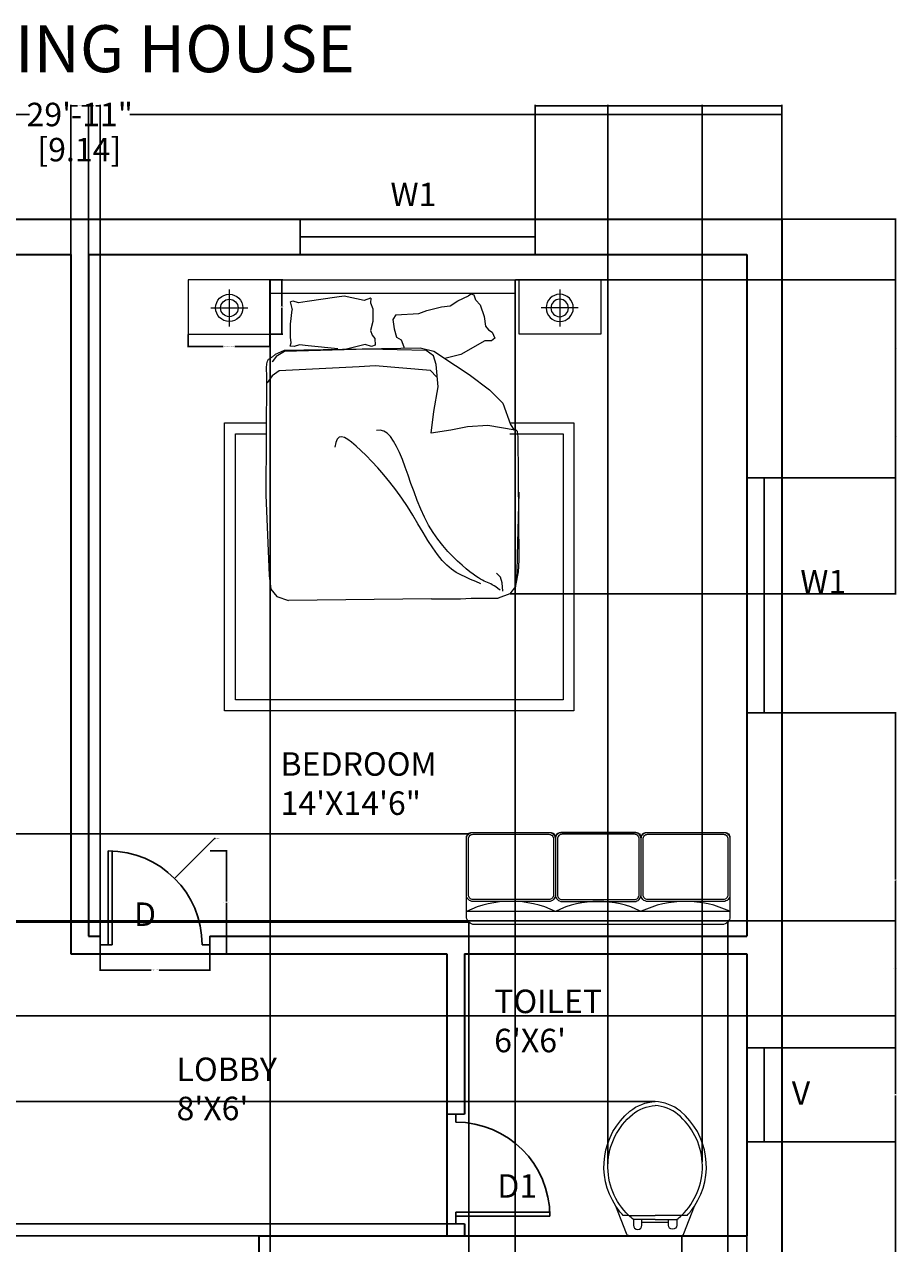
# Model space of a CAD drawing. Units: inches. Extents: x 3 to 420, y -502 to 54.
# Tile 6 of 6: x 198 to 420, y -257 to 54. Entities that reach past the tile are written whole.
import ezdxf

# ---------------------------------------------------------------- set-up
doc = ezdxf.new("R2010")
doc.units = ezdxf.units.IN
doc.header["$MEASUREMENT"] = 0
for name, color, linetype, lineweight in [('A-ANNO-DIMS', 2, 'Continuous', 18), ('A-ANNO-TEXT', 7, 'Continuous', 18), ('A-AREA-IDEN', 7, 'Continuous', 18), ('A-DOOR', 4, 'Continuous', 25), ('A-FURN', 8, 'Continuous', 18), ('A-GLAZ', 40, 'Continuous', 25), ('A-WALL', 7, 'Continuous', 35), ('WC-Detail_dwgmodels.com', 251, 'Continuous', 13), ('WC-Outline_dwgmodels.com', 250, 'Continuous', 18)]:
    doc.layers.add(name, color=color, linetype=linetype, lineweight=lineweight)
doc.styles.get("Standard").update_dxf_attribs({"font": 'arial.ttf'})
doc.dimstyles.get("Standard").update_dxf_attribs({"dimtxt": 0.18, "dimasz": 0.18, "dimexe": 0.18, "dimexo": 0.0625, "dimgap": 0.09, "dimtad": 0, "dimtih": 1, "dimtoh": 1, "dimdec": 0, "dimzin": 0, "dimdsep": 46, "dimlunit": 3, "dimtxsty": 'Standard', "dimcen": 0.09, "dimadec": 0, "dimazin": 0, "dimtfac": 1, "dimtdec": 0, "dimtofl": 0, "dimtmove": 0, "dimatfit": 3, "dimfxl": 1, "dimtolj": 1, "dimtzin": 0, "dimarcsym": 0})

# ---------------------------------------------------------------- blocks, each defined once
blk = doc.blocks.new('*D1')
at = {"layer": 'A-ANNO-DIMS', "color": 0, "lineweight": -2, "transparency": 16777216}
for p, q in [((32.39, 4.61), (32.39, 31.47)), ((32.57, 31.29), (198.86, 31.29)), ((390.71, 31.29), (224.42, 31.29)), ((390.89, 4.61), (390.89, 31.47))]:
    blk.add_line(p, q, dxfattribs=at)
at = {"layer": 'A-ANNO-DIMS', "color": 0, "transparency": 16777216}
for points in [[(32.57, 31.32), (32.57, 31.26), (32.39, 31.29)], [(390.71, 31.32), (390.71, 31.26), (390.89, 31.29)]]:
    blk.add_solid(points, dxfattribs=at)
at = {"layer": 'Defpoints', "color": 0, "transparency": 16777216}
for p in [(390.89, 31.29), (32.39, 4.54), (390.89, 4.54)]:
    blk.add_point(p, dxfattribs=at)
at = {"layer": 'A-ANNO-DIMS', "color": 0, "transparency": 16777216, "insert": (211.64, 31.29), "char_height": 6, "attachment_point": 5}
blk.add_mtext('\\A1;29\'-11"', dxfattribs=at)
blk = doc.blocks.new('DOOR-SWING-24')
for p, q in [((2, 2.25), (2, 26.25)), ((3, 2.25), (3, 26.25)), ((0, 4.5), (0, 0)), ((28, 2.25), (28, 4.5)), ((0, 2.25), (2, 2.25)), ((2, 2.25), (3, 2.25)), ((26, 2.25), (28, 2.25)), ((28, 2.25), (28, 0))]:
    blk.add_line(p, q)
blk.add_arc((2, 2.25), 24, 0, 90)
blk = doc.blocks.new('WIN-W1-60')
for p, q in [((0, 9), (60, 9)), ((0, 9), (0, 0)), ((60, 9), (60, 0)), ((0, 4.5), (60, 4.5)), ((0, 0), (60, 0))]:
    blk.add_line(p, q)
blk = doc.blocks.new('NIGHTSTAND-LARGE')
for p, q in [((10.53, 11.44), (10.53, 1.98)), ((5.81, 6.71), (15.26, 6.71))]:
    blk.add_line(p, q)
blk.add_lwpolyline([(0, 0), (20.85, 0), (20.85, 13.9), (0, 13.9)], close=True)
for radius in [3.48, 2.23]:
    blk.add_circle((10.53, 6.71), radius)
blk = doc.blocks.new('*D27')
at = {"layer": 'A-ANNO-DIMS', "color": 0, "lineweight": -2, "transparency": 16777216}
for p, q in [((216.89, -183.02), (216.89, -187.34)), ((244.89, -183.02), (244.89, -187.34)), ((217.07, -187.16), (229.84, -187.16)), ((244.71, -187.16), (231.94, -187.16))]:
    blk.add_line(p, q, dxfattribs=at)
at = {"layer": 'A-ANNO-DIMS', "color": 0, "transparency": 16777216}
for points in [[(217.07, -187.13), (217.07, -187.19), (216.89, -187.16)], [(244.71, -187.13), (244.71, -187.19), (244.89, -187.16)]]:
    blk.add_solid(points, dxfattribs=at)
at = {"layer": 'Defpoints', "color": 0, "transparency": 16777216}
for p in [(216.89, -182.96), (244.89, -182.96), (244.89, -187.16)]:
    blk.add_point(p, dxfattribs=at)
at = {"layer": 'A-ANNO-DIMS', "color": 0, "transparency": 16777216, "insert": (230.89, -187.16), "char_height": 0.18, "attachment_point": 5}
blk.add_mtext('\\A1;DOOR 2\'-4" TYP.', dxfattribs=at)
blk = doc.blocks.new('*D28')
at = {"layer": 'A-ANNO-DIMS', "color": 0, "lineweight": -2, "transparency": 16777216}
for p, q in [((244.95, -156.71), (249.27, -156.71)), ((249.09, -156.89), (249.09, -169.65)), ((249.09, -182.78), (249.09, -170.01)), ((244.95, -182.96), (249.27, -182.96))]:
    blk.add_line(p, q, dxfattribs=at)
at = {"layer": 'A-ANNO-DIMS', "color": 0, "transparency": 16777216}
for points in [[(249.06, -156.89), (249.12, -156.89), (249.09, -156.71)], [(249.06, -182.78), (249.12, -182.78), (249.09, -182.96)]]:
    blk.add_solid(points, dxfattribs=at)
at = {"layer": 'Defpoints', "color": 0, "transparency": 16777216}
for p in [(244.89, -156.71), (249.09, -156.71), (244.89, -182.96)]:
    blk.add_point(p, dxfattribs=at)
at = {"layer": 'A-ANNO-DIMS', "color": 0, "transparency": 16777216, "insert": (249.09, -169.83), "char_height": 0.18, "attachment_point": 5}
blk.add_mtext('\\A1;2\'-2 1/2" TYP.', dxfattribs=at)
blk = doc.blocks.new('*D29')
at = {"layer": 'A-ANNO-DIMS', "color": 0, "lineweight": -2, "transparency": 16777216}
for p, q in [((239.29, -24.87), (239.29, -28.11)), ((260.14, -24.87), (260.14, -28.11)), ((239.47, -27.93), (248.23, -27.93)), ((259.96, -27.93), (251.2, -27.93))]:
    blk.add_line(p, q, dxfattribs=at)
at = {"layer": 'A-ANNO-DIMS', "color": 0, "transparency": 16777216}
for points in [[(239.47, -27.9), (239.47, -27.96), (239.29, -27.93)], [(259.96, -27.9), (259.96, -27.96), (260.14, -27.93)]]:
    blk.add_solid(points, dxfattribs=at)
at = {"layer": 'Defpoints', "color": 0, "transparency": 16777216}
for p in [(239.29, -24.81), (260.14, -24.81), (260.14, -27.93)]:
    blk.add_point(p, dxfattribs=at)
at = {"layer": 'A-ANNO-DIMS', "color": 0, "transparency": 16777216, "insert": (249.71, -27.93), "char_height": 0.18, "attachment_point": 5}
blk.add_mtext('\\A1;NIGHTSTAND 1\'-9" TYP.', dxfattribs=at)
blk = doc.blocks.new('*D30')
at = {"layer": 'A-ANNO-DIMS', "color": 0, "lineweight": -2, "transparency": 16777216}
for p, q in [((260.2, -10.91), (263.45, -10.91)), ((263.27, -11.09), (263.27, -17.68)), ((263.27, -24.63), (263.27, -18.04)), ((260.2, -24.81), (263.45, -24.81))]:
    blk.add_line(p, q, dxfattribs=at)
at = {"layer": 'A-ANNO-DIMS', "color": 0, "transparency": 16777216}
for points in [[(263.24, -11.09), (263.3, -11.09), (263.27, -10.91)], [(263.24, -24.63), (263.3, -24.63), (263.27, -24.81)]]:
    blk.add_solid(points, dxfattribs=at)
at = {"layer": 'Defpoints', "color": 0, "transparency": 16777216}
for p in [(260.14, -10.91), (263.27, -10.91), (260.14, -24.81)]:
    blk.add_point(p, dxfattribs=at)
at = {"layer": 'A-ANNO-DIMS', "color": 0, "transparency": 16777216, "insert": (263.27, -17.86), "char_height": 0.18, "attachment_point": 5}
blk.add_mtext('\\A1;1\'-2" TYP.', dxfattribs=at)
blk = doc.blocks.new('*D49')
at = {"layer": 'A-ANNO-DIMS', "color": 0, "lineweight": -2, "transparency": 16777216}
for p, q in [((390.95, -206.96), (420.07, -206.96)), ((419.89, -207.14), (419.89, -218.77)), ((419.89, -230.78), (419.89, -219.14)), ((390.95, -230.96), (420.07, -230.96))]:
    blk.add_line(p, q, dxfattribs=at)
at = {"layer": 'A-ANNO-DIMS', "color": 0, "transparency": 16777216}
for points in [[(419.86, -207.14), (419.92, -207.14), (419.89, -206.96)], [(419.86, -230.78), (419.92, -230.78), (419.89, -230.96)]]:
    blk.add_solid(points, dxfattribs=at)
at = {"layer": 'Defpoints', "color": 0, "transparency": 16777216}
for p in [(390.89, -206.96), (390.89, -230.96), (419.89, -230.96)]:
    blk.add_point(p, dxfattribs=at)
at = {"layer": 'A-ANNO-DIMS', "color": 0, "transparency": 16777216, "insert": (419.89, -218.96), "char_height": 0.18, "attachment_point": 5}
blk.add_mtext('\\A1;2\'-0"', dxfattribs=at)
blk = doc.blocks.new('*D54')
at = {"layer": 'A-ANNO-DIMS', "color": 0, "lineweight": -2, "transparency": 16777216}
for p, q in [((327.89, 4.61), (327.89, 33.72)), ((328.07, 33.54), (359.06, 33.54)), ((390.71, 33.54), (359.72, 33.54)), ((390.89, 4.61), (390.89, 33.72))]:
    blk.add_line(p, q, dxfattribs=at)
at = {"layer": 'A-ANNO-DIMS', "color": 0, "transparency": 16777216}
for points in [[(328.07, 33.57), (328.07, 33.51), (327.89, 33.54)], [(390.71, 33.57), (390.71, 33.51), (390.89, 33.54)]]:
    blk.add_solid(points, dxfattribs=at)
at = {"layer": 'Defpoints', "color": 0, "transparency": 16777216}
for p in [(390.89, 33.54), (327.89, 4.54), (390.89, 4.54)]:
    blk.add_point(p, dxfattribs=at)
at = {"layer": 'A-ANNO-DIMS', "color": 0, "transparency": 16777216, "insert": (359.39, 33.54), "char_height": 0.18, "attachment_point": 5}
blk.add_mtext('\\A1;5\'-3"', dxfattribs=at)
blk = doc.blocks.new('*D55')
at = {"layer": 'A-ANNO-DIMS', "color": 0, "lineweight": -2, "transparency": 16777216}
for p, q in [((390.95, 4.54), (420.07, 4.54)), ((419.89, 4.36), (419.89, -28.27)), ((419.89, -61.28), (419.89, -28.64)), ((390.95, -61.46), (420.07, -61.46))]:
    blk.add_line(p, q, dxfattribs=at)
at = {"layer": 'A-ANNO-DIMS', "color": 0, "transparency": 16777216}
for points in [[(419.86, 4.36), (419.92, 4.36), (419.89, 4.54)], [(419.86, -61.28), (419.92, -61.28), (419.89, -61.46)]]:
    blk.add_solid(points, dxfattribs=at)
at = {"layer": 'Defpoints', "color": 0, "transparency": 16777216}
for p in [(390.89, 4.54), (390.89, -61.46), (419.89, -61.46)]:
    blk.add_point(p, dxfattribs=at)
at = {"layer": 'A-ANNO-DIMS', "color": 0, "transparency": 16777216, "insert": (419.89, -28.46), "char_height": 0.18, "attachment_point": 5}
blk.add_mtext('\\A1;5\'-6"', dxfattribs=at)
blk = doc.blocks.new('*D56')
at = {"layer": 'A-ANNO-DIMS', "color": 0, "lineweight": -2, "transparency": 16777216}
for p, q in [((390.95, -121.46), (420.07, -121.46)), ((419.89, -121.64), (419.89, -164.02)), ((419.89, -206.78), (419.89, -164.39)), ((390.95, -206.96), (420.07, -206.96))]:
    blk.add_line(p, q, dxfattribs=at)
at = {"layer": 'A-ANNO-DIMS', "color": 0, "transparency": 16777216}
for points in [[(419.86, -121.64), (419.92, -121.64), (419.89, -121.46)], [(419.86, -206.78), (419.92, -206.78), (419.89, -206.96)]]:
    blk.add_solid(points, dxfattribs=at)
at = {"layer": 'Defpoints', "color": 0, "transparency": 16777216}
for p in [(390.89, -121.46), (390.89, -206.96), (419.89, -206.96)]:
    blk.add_point(p, dxfattribs=at)
at = {"layer": 'A-ANNO-DIMS', "color": 0, "transparency": 16777216, "insert": (419.89, -164.21), "char_height": 0.18, "attachment_point": 5}
blk.add_mtext('\\A1;7\'-1 1/2"', dxfattribs=at)
blk = doc.blocks.new('*D57')
at = {"layer": 'A-ANNO-DIMS', "color": 0, "lineweight": -2, "transparency": 16777216}
for p, q in [((390.95, -230.96), (420.07, -230.96)), ((419.89, -231.14), (419.89, -260.02)), ((419.89, -289.28), (419.89, -260.39)), ((390.95, -289.46), (420.07, -289.46))]:
    blk.add_line(p, q, dxfattribs=at)
at = {"layer": 'A-ANNO-DIMS', "color": 0, "transparency": 16777216}
for points in [[(419.86, -231.14), (419.92, -231.14), (419.89, -230.96)], [(419.86, -289.28), (419.92, -289.28), (419.89, -289.46)]]:
    blk.add_solid(points, dxfattribs=at)
at = {"layer": 'Defpoints', "color": 0, "transparency": 16777216}
for p in [(390.89, -230.96), (390.89, -289.46), (419.89, -289.46)]:
    blk.add_point(p, dxfattribs=at)
at = {"layer": 'A-ANNO-DIMS', "color": 0, "transparency": 16777216, "insert": (419.89, -260.21), "char_height": 0.18, "attachment_point": 5}
blk.add_mtext('\\A1;4\'-10 1/2"', dxfattribs=at)
blk = doc.blocks.new('*D64')
at = {"layer": 'A-ANNO-DIMS', "color": 0, "lineweight": -2, "transparency": 16777216}
for p, q in [((209.39, -4.39), (209.39, 33.72)), ((209.57, 33.54), (211.1, 33.54)), ((213.71, 33.54), (212.18, 33.54)), ((213.89, -4.39), (213.89, 33.72))]:
    blk.add_line(p, q, dxfattribs=at)
at = {"layer": 'A-ANNO-DIMS', "color": 0, "transparency": 16777216}
for points in [[(209.57, 33.57), (209.57, 33.51), (209.39, 33.54)], [(213.71, 33.57), (213.71, 33.51), (213.89, 33.54)]]:
    blk.add_solid(points, dxfattribs=at)
at = {"layer": 'Defpoints', "color": 0, "transparency": 16777216}
for p in [(213.89, 33.54), (209.39, -4.46), (213.89, -4.46)]:
    blk.add_point(p, dxfattribs=at)
at = {"layer": 'A-ANNO-DIMS', "color": 0, "transparency": 16777216, "insert": (211.64, 33.54), "char_height": 0.18, "attachment_point": 5}
blk.add_mtext('\\A1;0\'-4 1/2"', dxfattribs=at)
blk = doc.blocks.new('*D65')
at = {"layer": 'A-ANNO-DIMS', "color": 0, "lineweight": -2, "transparency": 16777216}
for p, q in [((260.22, -10.97), (260.22, -501.64)), ((322.8, -10.97), (322.8, -501.64)), ((260.4, -501.46), (290.97, -501.46)), ((322.62, -501.46), (292.05, -501.46))]:
    blk.add_line(p, q, dxfattribs=at)
at = {"layer": 'A-ANNO-DIMS', "color": 0, "transparency": 16777216}
for points in [[(260.4, -501.43), (260.4, -501.49), (260.22, -501.46)], [(322.62, -501.43), (322.62, -501.49), (322.8, -501.46)]]:
    blk.add_solid(points, dxfattribs=at)
at = {"layer": 'Defpoints', "color": 0, "transparency": 16777216}
for p in [(260.22, -10.9), (322.8, -10.9), (322.8, -501.46)]:
    blk.add_point(p, dxfattribs=at)
at = {"layer": 'A-ANNO-DIMS', "color": 0, "transparency": 16777216, "insert": (291.51, -501.46), "char_height": 0.18, "attachment_point": 5}
blk.add_mtext('\\A1;5\'-2 1/2"', dxfattribs=at)
blk = doc.blocks.new('*D66')
at = {"layer": 'A-ANNO-DIMS', "color": 0, "lineweight": -2, "transparency": 16777216}
for p, q in [((322.86, -10.9), (420.07, -10.9)), ((419.89, -11.08), (419.89, -50.81)), ((419.89, -90.91), (419.89, -51.18)), ((321.49, -91.09), (420.07, -91.09))]:
    blk.add_line(p, q, dxfattribs=at)
at = {"layer": 'A-ANNO-DIMS', "color": 0, "transparency": 16777216}
for points in [[(419.86, -11.08), (419.92, -11.08), (419.89, -10.9)], [(419.86, -90.91), (419.92, -90.91), (419.89, -91.09)]]:
    blk.add_solid(points, dxfattribs=at)
at = {"layer": 'Defpoints', "color": 0, "transparency": 16777216}
for p in [(322.8, -10.9), (321.42, -91.09), (419.89, -91.09)]:
    blk.add_point(p, dxfattribs=at)
at = {"layer": 'A-ANNO-DIMS', "color": 0, "transparency": 16777216, "insert": (419.89, -51), "char_height": 0.18, "attachment_point": 5}
blk.add_mtext('\\A1;6\'-8"', dxfattribs=at)
blk = doc.blocks.new('*D69')
at = {"layer": 'A-ANNO-DIMS', "color": 0, "lineweight": -2, "transparency": 16777216}
for p, q in [((310.96, -174.99), (310.96, -501.64)), ((377.04, -174.99), (377.04, -501.64)), ((311.14, -501.46), (343.67, -501.46)), ((376.86, -501.46), (344.33, -501.46))]:
    blk.add_line(p, q, dxfattribs=at)
at = {"layer": 'A-ANNO-DIMS', "color": 0, "transparency": 16777216}
for points in [[(311.14, -501.43), (311.14, -501.49), (310.96, -501.46)], [(376.86, -501.43), (376.86, -501.49), (377.04, -501.46)]]:
    blk.add_solid(points, dxfattribs=at)
at = {"layer": 'Defpoints', "color": 0, "transparency": 16777216}
for p in [(310.96, -174.93), (377.04, -174.93), (377.04, -501.46)]:
    blk.add_point(p, dxfattribs=at)
at = {"layer": 'A-ANNO-DIMS', "color": 0, "transparency": 16777216, "insert": (344, -501.46), "char_height": 0.18, "attachment_point": 5}
blk.add_mtext('\\A1;5\'-6"', dxfattribs=at)
blk = doc.blocks.new('*D70')
at = {"layer": 'A-ANNO-DIMS', "color": 0, "lineweight": -2, "transparency": 16777216}
for p, q in [((310.7, -152.37), (3.21, -152.37)), ((3.39, -152.55), (3.39, -163.47)), ((3.39, -174.75), (3.39, -163.83)), ((310.9, -174.93), (3.21, -174.93))]:
    blk.add_line(p, q, dxfattribs=at)
at = {"layer": 'A-ANNO-DIMS', "color": 0, "transparency": 16777216}
for points in [[(3.36, -152.55), (3.42, -152.55), (3.39, -152.37)], [(3.36, -174.75), (3.42, -174.75), (3.39, -174.93)]]:
    blk.add_solid(points, dxfattribs=at)
at = {"layer": 'Defpoints', "color": 0, "transparency": 16777216}
for p in [(3.39, -152.37), (310.77, -152.37), (310.96, -174.93)]:
    blk.add_point(p, dxfattribs=at)
at = {"layer": 'A-ANNO-DIMS', "color": 0, "transparency": 16777216, "insert": (3.39, -163.65), "char_height": 0.18, "attachment_point": 5}
blk.add_mtext('\\A1;1\'-10 1/2"', dxfattribs=at)
blk = doc.blocks.new('*D72')
at = {"layer": 'A-ANNO-DIMS', "color": 0, "lineweight": -2, "transparency": 16777216}
for p, q in [((138.83, -174.56), (420.07, -174.56)), ((419.89, -174.74), (419.89, -186.51)), ((419.89, -198.65), (419.89, -186.87)), ((138.83, -198.83), (420.07, -198.83))]:
    blk.add_line(p, q, dxfattribs=at)
at = {"layer": 'A-ANNO-DIMS', "color": 0, "transparency": 16777216}
for points in [[(419.86, -174.74), (419.92, -174.74), (419.89, -174.56)], [(419.86, -198.65), (419.92, -198.65), (419.89, -198.83)]]:
    blk.add_solid(points, dxfattribs=at)
at = {"layer": 'Defpoints', "color": 0, "transparency": 16777216}
for p in [(138.77, -174.56), (138.77, -198.83), (419.89, -198.83)]:
    blk.add_point(p, dxfattribs=at)
at = {"layer": 'A-ANNO-DIMS', "color": 0, "transparency": 16777216, "insert": (419.89, -186.69), "char_height": 0.18, "attachment_point": 5}
blk.add_mtext('\\A1;2\'-0 1/2"', dxfattribs=at)
blk = doc.blocks.new('*D75')
at = {"layer": 'A-ANNO-DIMS', "color": 0, "lineweight": -2, "transparency": 16777216}
for p, q in [((346.48, -236.6), (346.48, 33.72)), ((346.66, 33.54), (358.18, 33.54)), ((370.37, 33.54), (358.84, 33.54)), ((370.55, -236.11), (370.55, 33.72))]:
    blk.add_line(p, q, dxfattribs=at)
at = {"layer": 'A-ANNO-DIMS', "color": 0, "transparency": 16777216}
for points in [[(346.66, 33.57), (346.66, 33.51), (346.48, 33.54)], [(370.37, 33.57), (370.37, 33.51), (370.55, 33.54)]]:
    blk.add_solid(points, dxfattribs=at)
at = {"layer": 'Defpoints', "color": 0, "transparency": 16777216}
for p in [(370.55, 33.54), (370.55, -236.17), (346.48, -236.66)]:
    blk.add_point(p, dxfattribs=at)
at = {"layer": 'A-ANNO-DIMS', "color": 0, "transparency": 16777216, "insert": (358.51, 33.54), "char_height": 0.18, "attachment_point": 5}
blk.add_mtext('\\A1;2\'-0"', dxfattribs=at)
blk = doc.blocks.new('*D76')
at = {"layer": 'A-ANNO-DIMS', "color": 0, "lineweight": -2, "transparency": 16777216}
for p, q in [((358.46, -220.72), (3.21, -220.72)), ((3.39, -220.9), (3.39, -237.66)), ((3.39, -254.78), (3.39, -238.02)), ((365, -254.96), (3.21, -254.96))]:
    blk.add_line(p, q, dxfattribs=at)
at = {"layer": 'A-ANNO-DIMS', "color": 0, "transparency": 16777216}
for points in [[(3.36, -220.9), (3.42, -220.9), (3.39, -220.72)], [(3.36, -254.78), (3.42, -254.78), (3.39, -254.96)]]:
    blk.add_solid(points, dxfattribs=at)
at = {"layer": 'Defpoints', "color": 0, "transparency": 16777216}
for p in [(358.53, -220.72), (3.39, -254.96), (365.06, -254.96)]:
    blk.add_point(p, dxfattribs=at)
at = {"layer": 'A-ANNO-DIMS', "color": 0, "transparency": 16777216, "insert": (3.39, -237.84), "char_height": 0.18, "attachment_point": 5}
blk.add_mtext('\\A1;2\'-10"', dxfattribs=at)
blk = doc.blocks.new('*D77')
at = {"layer": 'A-ANNO-DIMS', "color": 0, "lineweight": -2, "transparency": 16777216}
for p, q in [((365.32, -254.98), (365.32, -501.64)), ((381.89, -255.02), (381.89, -501.64)), ((365.5, -501.46), (373.07, -501.46)), ((381.71, -501.46), (374.14, -501.46))]:
    blk.add_line(p, q, dxfattribs=at)
at = {"layer": 'A-ANNO-DIMS', "color": 0, "transparency": 16777216}
for points in [[(365.5, -501.43), (365.5, -501.49), (365.32, -501.46)], [(381.71, -501.43), (381.71, -501.49), (381.89, -501.46)]]:
    blk.add_solid(points, dxfattribs=at)
at = {"layer": 'Defpoints', "color": 0, "transparency": 16777216}
for p in [(365.32, -254.92), (381.89, -254.96), (381.89, -501.46)]:
    blk.add_point(p, dxfattribs=at)
at = {"layer": 'A-ANNO-DIMS', "color": 0, "transparency": 16777216, "insert": (373.6, -501.46), "char_height": 0.18, "attachment_point": 5}
blk.add_mtext('\\A1;1\'-4 1/2"', dxfattribs=at)
blk = doc.blocks.new('*D80')
at = {"layer": 'A-ANNO-DIMS', "color": 0, "lineweight": -2, "transparency": 16777216}
for p, q in [((213.89, -178.39), (213.89, 33.72)), ((214.07, 33.54), (215.06, 33.54)), ((216.71, 33.54), (215.72, 33.54)), ((216.89, -178.39), (216.89, 33.72))]:
    blk.add_line(p, q, dxfattribs=at)
at = {"layer": 'A-ANNO-DIMS', "color": 0, "transparency": 16777216}
for points in [[(214.07, 33.57), (214.07, 33.51), (213.89, 33.54)], [(216.71, 33.57), (216.71, 33.51), (216.89, 33.54)]]:
    blk.add_solid(points, dxfattribs=at)
at = {"layer": 'Defpoints', "color": 0, "transparency": 16777216}
for p in [(216.89, 33.54), (213.89, -178.46), (216.89, -178.46)]:
    blk.add_point(p, dxfattribs=at)
at = {"layer": 'A-ANNO-DIMS', "color": 0, "transparency": 16777216, "insert": (215.39, 33.54), "char_height": 0.18, "attachment_point": 5}
blk.add_mtext('\\A1;0\'-3"', dxfattribs=at)
blk = doc.blocks.new('*D81')
at = {"layer": 'A-ANNO-DIMS', "color": 0, "lineweight": -2, "transparency": 16777216}
for p, q in [((309.83, -251.96), (3.21, -251.96)), ((309.83, -254.96), (3.21, -254.96)), ((3.39, -252.14), (3.39, -253.27)), ((3.39, -254.78), (3.39, -253.64))]:
    blk.add_line(p, q, dxfattribs=at)
at = {"layer": 'A-ANNO-DIMS', "color": 0, "transparency": 16777216}
for points in [[(3.36, -252.14), (3.42, -252.14), (3.39, -251.96)], [(3.36, -254.78), (3.42, -254.78), (3.39, -254.96)]]:
    blk.add_solid(points, dxfattribs=at)
at = {"layer": 'Defpoints', "color": 0, "transparency": 16777216}
for p in [(309.89, -251.96), (3.39, -254.96), (309.89, -254.96)]:
    blk.add_point(p, dxfattribs=at)
at = {"layer": 'A-ANNO-DIMS', "color": 0, "transparency": 16777216, "insert": (3.39, -253.46), "char_height": 0.18, "attachment_point": 5}
blk.add_mtext('\\A1;0\'-3"', dxfattribs=at)
blk = doc.blocks.new('*D84')
at = {"layer": 'A-ANNO-DIMS', "color": 0, "lineweight": -2, "transparency": 16777216}
for p, q in [((246.04, -153.55), (235.99, -163.61)), ((246.22, -153.55), (246.04, -153.55)), ((218.8, -180.71), (218.98, -180.71)), ((218.89, -180.8), (218.89, -180.62))]:
    blk.add_line(p, q, dxfattribs=at)
at = {"layer": 'A-ANNO-DIMS', "color": 0, "transparency": 16777216}
blk.add_solid([(235.97, -163.59), (236.01, -163.63), (235.86, -163.74)], dxfattribs=at)
at = {"layer": 'Defpoints', "color": 0, "transparency": 16777216}
for p in [(235.86, -163.74), (218.89, -180.71)]:
    blk.add_point(p, dxfattribs=at)
at = {"layer": 'A-ANNO-DIMS', "color": 0, "transparency": 16777216, "insert": (246.83, -153.55), "char_height": 0.18, "attachment_point": 5}
blk.add_mtext('\\A1;3X R2\'-0"', dxfattribs=at)

msp = doc.modelspace()

# ---------------------------------------------------------------- linework, layer by layer
at = {"layer": 'A-FURN'}
for p, q in [((260.22, -31.02), (260.22, -10.9)), ((279.13, -15.11), (277.23, -15.32)), ((284.25, -16.18), (279.13, -15.11)), ((308.13, -16.29), (310.89, -15.01)), ((265.97, -18.56), (265.44, -16.54)), ((285.83, -15.6), (284.25, -16.18)), ((285.98, -15.64), (285.83, -15.6)), ((285.98, -15.64), (285.86, -16.81)), ((285.98, -15.64), (285.86, -16.81)), ((285.86, -16.81), (286.49, -18.32)), ((286.49, -18.32), (286.47, -21.52)), ((300.22, -18.79), (303.98, -17.78)), ((303.98, -17.78), (306.18, -17.59)), ((306.18, -17.59), (308.13, -16.29)), ((306.18, -17.59), (308.13, -16.29)), ((312.76, -16.09), (313.87, -17.3)), ((313.87, -17.3), (314.92, -20.32)), ((286.47, -21.52), (285.89, -23.88)), ((292.35, -19.89), (298.22, -19.54)), ((298.22, -19.54), (300.22, -18.79)), ((314.92, -20.32), (315.19, -22.74)), ((285.89, -23.88), (286.29, -25.02)), ((315.19, -22.74), (315.95, -23.67)), ((315.95, -23.67), (316.91, -24.28)), ((316.91, -24.28), (317.57, -25.82)), ((284.5, -27.4), (279.43, -28.7)), ((286.11, -27.91), (284.5, -27.4)), ((287.09, -27.59), (286.11, -27.91)), ((286.29, -25.02), (286.99, -25.92)), ((286.99, -25.92), (287.09, -27.59)), ((315.07, -26.52), (308.9, -29.98)), ((316.75, -26.46), (315.07, -26.52)), ((317.57, -25.82), (316.75, -26.46)), ((259.34, -32.4), (259.25, -33.37)), ((259.25, -33.37), (259.28, -35.64)), ((259.28, -35.64), (259.15, -65.92)), ((322.69, -49.3), (322.82, -49.24)), ((323.62, -60.95), (323.52, -51.12)), ((323.84, -82.46), (323.62, -60.95)), ((323.69, -65.16), (323.27, -81.42)), ((259.15, -65.92), (259.8, -82.16)), ((259.8, -82.16), (260.03, -86.41)), ((323.27, -81.42), (323.18, -85.68)), ((323.66, -85.45), (323.84, -82.46)), ((260.03, -86.41), (260.41, -89.91)), ((319.05, -86.87), (318.03, -85.81)), ((319.51, -88.3), (319.05, -86.87)), ((323.18, -85.68), (322.9, -89.19)), ((323.08, -88.55), (323.66, -85.45)), ((260.41, -89.91), (261.94, -91.77)), ((319.61, -90.37), (319.51, -88.3)), ((322.9, -89.19), (321.42, -91.09)), ((261.94, -91.77), (264.91, -92.77)), ((301.42, -92.37), (264.91, -92.77)), ((301.42, -92.37), (308.88, -92.37)), ((308.88, -92.37), (311.52, -92.18)), ((311.52, -92.18), (318.49, -92.17)), ((321.42, -91.09), (318.49, -92.17))]:
    msp.add_line(p, q, dxfattribs=at)
for points in [[(260.22, -10.9), (322.8, -10.9), (322.8, -49.19)], [(322.8, -14.38), (260.22, -14.38)], [(277.23, -15.32), (269.66, -16.46), (267.47, -16.83), (266.16, -16.41), (265.44, -16.54)], [(312.76, -16.09), (312.37, -14.81), (311.54, -14.55), (310.89, -15.01)], [(277.53, -28.58), (269.92, -27.78), (267.71, -27.51), (266.42, -27.98), (265.36, -27.85), (265.65, -27.01), (265.47, -25.56), (265.42, -22.22), (265.9, -18.56)], [(292.35, -19.89), (291.54, -21.04), (291.93, -23.46), (292.51, -25.58), (293.67, -26.26), (294.34, -28), (294.35, -28.32)], [(259.37, -32.34), (259.57, -31.69), (259.87, -31.19), (260.22, -31.02), (260.63, -30.66), (260.69, -30.64)], [(322.8, -49.33), (315.78, -48.1), (310.61, -48.49), (306.38, -49.34), (301.36, -50.05), (302.04, -44.57), (303.17, -38.2), (302.67, -32.58), (301.94, -30.3), (300.1, -29), (285.27, -28.59), (263.95, -29.23), (261.77, -30.52), (260.85, -31.79), (260.73, -31.91)], [(260.75, -30.65), (261.6, -29.9), (263.95, -28.92), (298.52, -28.24), (301.99, -29.13), (307.54, -32.82), (311.03, -35.12), (316.27, -38.97), (319.62, -42.38), (321.59, -47.85), (322.56, -49.29)], [(308.9, -29.98), (304.8, -30.99)], [(302.75, -35.68), (301.18, -34.08), (287.06, -32.89), (282.95, -33.13), (262.52, -34.15), (260.8, -35.45), (259.5, -37.19)], [(321.45, -47.46), (337.81, -47.46), (337.81, -120.93), (248.6, -120.93), (248.6, -47.46), (259.23, -47.46)], [(318.99, -90.14), (318.41, -89.7), (317.88, -89.34), (317.4, -89.04), (316.96, -88.79), (316.54, -88.57), (316.13, -88.38), (315.73, -88.21), (315.33, -88.03), (314.91, -87.84), (314.46, -87.61), (313.96, -87.34), (313.41, -87.01), (312.78, -86.59), (312.07, -86.08), (311.25, -85.45), (310.32, -84.7), (309.26, -83.8), (308.11, -82.76), (306.88, -81.57), (305.61, -80.24), (304.33, -78.77), (303.06, -77.17), (301.84, -75.42), (300.69, -73.55), (299.64, -71.54), (298.68, -69.43), (297.8, -67.27), (296.98, -65.08), (296.2, -62.9), (295.46, -60.77), (294.73, -58.72), (294, -56.79), (293.26, -55.03), (292.51, -53.44), (291.73, -52.07), (290.93, -50.94), (290.09, -50.08), (289.23, -49.52), (288.32, -49.27), (287.37, -49.38)], [(323.52, -51.03), (323.42, -49.68), (323.03, -49.27), (322.8, -49.19)], [(321.45, -50.24), (335.03, -50.24), (335.03, -118.15), (251.38, -118.15), (251.38, -50.24), (259.23, -50.24)], [(314.05, -88.5), (312.72, -87.92), (311.43, -87.39), (310.17, -86.85), (308.94, -86.27), (307.73, -85.6), (306.53, -84.78), (305.34, -83.79), (304.15, -82.56), (302.96, -81.07), (301.75, -79.35), (300.52, -77.44), (299.27, -75.39), (297.98, -73.24), (296.65, -71.04), (295.27, -68.83), (293.84, -66.66), (292.34, -64.57), (290.81, -62.57), (289.26, -60.68), (287.73, -58.92), (286.22, -57.29), (284.78, -55.81), (283.42, -54.49), (282.17, -53.35), (281.05, -52.4), (280.06, -51.67), (279.19, -51.19), (278.46, -51), (277.84, -51.11), (277.35, -51.58), (276.98, -52.42), (276.73, -53.66)], [(377.63, -172.15), (310.37, -172.15)]]:
    msp.add_lwpolyline(points, dxfattribs=at)
for points in [[(333.07, -153.66), (333.07, -167.95, -0.414214), (331.39, -169.63), (312.05, -169.63, -0.414214), (310.37, -167.95), (310.37, -153.66, -0.414214), (312.05, -151.98), (331.39, -151.98, -0.414214)], [(332.57, -153.66), (332.57, -167.95, -0.414214), (331.39, -169.13), (312.05, -169.13, -0.414214), (310.88, -167.95), (310.88, -153.66, -0.414214), (312.05, -152.48), (331.39, -152.48, -0.414214)], [(333.07, -153.66), (333.07, -167.95, 0.414214), (334.75, -169.63), (353.25, -169.63, 0.414214), (354.93, -167.95), (354.93, -153.66, 0.414214), (353.25, -151.98), (334.75, -151.98, 0.414214)], [(333.58, -153.66), (333.58, -167.95, 0.414214), (334.75, -169.13), (353.25, -169.13, 0.414214), (354.43, -167.95), (354.43, -153.66, 0.414214), (353.25, -152.48), (334.75, -152.48, 0.414214)], [(377.63, -153.66), (377.63, -167.95, -0.414214), (375.95, -169.63), (356.61, -169.63, -0.414214), (354.93, -167.95), (354.93, -153.66, -0.414214), (356.61, -151.98), (375.95, -151.98, -0.414214)], [(377.12, -153.66), (377.12, -167.95, -0.414214), (375.95, -169.13), (356.61, -169.13, -0.414214), (355.43, -167.95), (355.43, -153.66, -0.414214), (356.61, -152.48), (375.95, -152.48, -0.414214)]]:
    msp.add_lwpolyline(points, format="xyb", close=True, dxfattribs=at)
at = {"layer": 'A-FURN', "ltscale": 0.03}
msp.add_lwpolyline([(356.29, -151.98), (376.28, -151.98, -0.414214), (377.63, -153.32), (377.63, -173.5, -0.414214), (375.61, -175.52), (312.39, -175.52, -0.414214), (310.37, -173.5), (310.37, -153.32, -0.414214), (311.72, -151.98), (331.71, -151.98, -0.414214), (333.06, -153.32, 1), (333.09, -153.32, -0.414214), (334.43, -151.98), (353.57, -151.98, -0.414214), (354.91, -153.32, 1), (354.95, -153.32, -0.414214)], format="xyb", close=True, dxfattribs=at)
at = {"layer": 'A-FURN'}
for centre, radius, start, end in [((321.72, -196.11), 26.51, 64.6538, 115.3462), ((344, -194.43), 24.82, 63.869, 116.131), ((366.28, -196.39), 26.77, 64.9106, 115.0894)]:
    msp.add_arc(centre, radius, start, end, dxfattribs=at)
at = {"layer": 'A-GLAZ'}
for p, q in [((381.89, -206.96), (381.89, -230.96)), ((390.89, -206.96), (381.89, -206.96)), ((386.39, -206.96), (386.39, -230.96)), ((390.89, -230.96), (390.89, -206.96)), ((381.89, -230.96), (390.89, -230.96))]:
    msp.add_line(p, q, dxfattribs=at)
at = {"layer": 'A-WALL'}
for p, q in [((32.39, 4.54), (390.89, 4.54)), ((390.89, 4.54), (390.89, -472.46)), ((41.39, -4.46), (209.39, -4.46)), ((209.39, -4.46), (209.39, -182.96)), ((213.89, -4.46), (213.89, -178.46)), ((213.89, -4.46), (381.89, -4.46)), ((381.89, -4.46), (381.89, -178.46)), ((213.89, -178.46), (216.89, -178.46)), ((244.89, -178.46), (381.89, -178.46)), ((209.39, -182.96), (305.39, -182.96)), ((305.39, -182.96), (305.39, -254.96)), ((309.89, -182.96), (309.89, -223.96)), ((309.89, -182.96), (381.89, -182.96)), ((381.89, -182.96), (381.89, -254.96)), ((309.89, -251.96), (309.89, -254.96)), ((257.39, -254.96), (381.89, -254.96)), ((257.39, -254.96), (257.39, -383.96))]:
    msp.add_line(p, q, dxfattribs=at)
at = {"layer": 'WC-Detail_dwgmodels.com'}
for p, q in [((351.79, -249.77), (350.35, -249.77)), ((366.7, -249.77), (365.26, -249.77))]:
    msp.add_line(p, q, dxfattribs=at)
for points in [[(350.35, -249.77, -0.040937), (348.5, -247.42, -0.163732)], [(366.7, -249.77, 0.040937), (368.55, -247.42, 0.163732)], [(352.97, -250.81, -0.022712), (351.79, -249.77, -0.162618)], [(358.53, -250.81), (352.97, -250.81, -0.476108)], [(352.97, -250.81), (352.97, -252.24, 1), (355.16, -252.24), (355.16, -251.5)], [(358.53, -250.81), (364.08, -250.81, 0.022712)], [(364.08, -250.81), (364.08, -252.24, -1), (361.9, -252.24), (361.9, -251.5)], [(364.08, -250.81, 0.022712), (365.26, -249.77, 0.162618)]]:
    msp.add_lwpolyline(points, format="xyb", dxfattribs=at)
for points in [[(355.16, -251.5), (355.16, -250.81)], [(355.16, -251.5), (361.9, -251.5)], [(361.9, -251.5), (361.9, -250.81)]]:
    msp.add_lwpolyline(points, dxfattribs=at)
at = {"layer": 'WC-Outline_dwgmodels.com'}
for p in [(351.79, -249.77), (365.26, -249.77)]:
    msp.add_line(p, (358.53, -249.77), dxfattribs=at)
for points in [[(348.5, -247.42, -0.383919), (352.09, -223.19, -0.163732), (358.53, -220.72, -0.359733)], [(368.55, -247.42, 0.383919), (364.96, -223.19, 0.163732), (358.53, -220.72, 0.359733)], [(351.79, -249.77, -0.448546), (352.74, -223.98, -0.162618), (358.53, -221.75, -0.470877)], [(365.95, -249.08, 0.431639), (364.31, -223.98, 0.162618), (358.53, -221.75, 0.470877)], [(358.53, -254.96), (351.99, -254.96, -0.31031), (351.19, -254.41), (348.5, -247.42, -0.209071)], [(358.53, -254.96), (365.06, -254.96, 0.31031), (365.86, -254.41), (368.55, -247.42, 0.209071)], [(365.26, -249.77, 0.014165), (365.95, -249.08, 0.162618)]]:
    msp.add_lwpolyline(points, format="xyb", dxfattribs=at)

# ---------------------------------------------------------------- block references
at = {"layer": 'A-DOOR'}
msp.add_blockref('DOOR-SWING-24', (216.89, -182.96), dxfattribs=at)
at = {"layer": 'A-DOOR', "extrusion": (0, 0, -1), "zscale": -1, "rotation": 90.00000000000003}
msp.add_blockref('DOOR-SWING-24', (-305.39, -251.96), dxfattribs=at)
at = {"layer": 'A-FURN'}
msp.add_blockref('NIGHTSTAND-LARGE', (239.29, -24.81), dxfattribs=at)
at = {"layer": 'A-FURN', "extrusion": (0, 0, -1), "zscale": -1}
msp.add_blockref('NIGHTSTAND-LARGE', (-344.69, -24.81), dxfattribs=at)
at = {"layer": 'A-GLAZ'}
for p, rotation in [((327.89, 4.54), 180), ((381.89, -61.46), 270)]:
    msp.add_blockref('WIN-W1-60', p, dxfattribs=dict(at, rotation=rotation))

# ---------------------------------------------------------------- texts
at = {"layer": 'A-ANNO-DIMS', "insert": (200.82, 25.32), "char_height": 6, "attachment_point": 1}
msp.add_mtext('[9.14]', dxfattribs=at)
at = {"layer": 'A-ANNO-TEXT', "attachment_point": 1}
for s, insert, char_height in [('NORTH FACING HOUSE', (105.86, 54.08), 12), ('W1', (290.96, 13.89), 6), ('W1', (395.57, -84.96), 6), ('D', (225.49, -169.88), 6), ('V', (393.39, -215.52), 6), ('D1', (318.23, -239.25), 6)]:
    msp.add_mtext(s, dxfattribs=dict(at, insert=insert, char_height=char_height))
at = {"layer": 'A-AREA-IDEN', "char_height": 6, "attachment_point": 1}
for s, insert in [('BEDROOM\\P14\'X14\'6"', (262.91, -131.53)), ("TOILET\\P6'X6'", (317.44, -192.13)), ("LOBBY\\P8'X6'", (236.36, -209.48))]:
    msp.add_mtext(s, dxfattribs=dict(at, insert=insert))

# ---------------------------------------------------------------- dimensions: what is measured, and where the dimension line sits
at = {"layer": 'A-ANNO-DIMS'}
for base, p1, p2, override, picture, middle in [((390.88918496, 31.29388447), (32.38918496, 4.54371834), (390.88918496, 4.54371834), {"dimtxt": 6, "dimclrd": 0, "dimclre": 0, "dimclrt": 0}, '*D1', (211.63918496, 31.29388447)), ((213.89, 33.54), (209.39, -4.46), (213.89, -4.46), {"dimdec": 1, "dimlfac": 1, "dimrnd": 0, "dimzin": 1, "dimdsep": 46, "dimlunit": 4, "dimfrac": 2}, '*D64', (211.64, 33.54)), ((216.89, 33.54), (213.89, -178.46), (216.89, -178.46), {"dimdec": 1, "dimlfac": 1, "dimrnd": 0, "dimzin": 1, "dimdsep": 46, "dimlunit": 4, "dimfrac": 2}, '*D80', (215.39, 33.54)), ((390.89, 33.54), (327.89, 4.54), (390.89, 4.54), {"dimdec": 1, "dimlfac": 1, "dimrnd": 0, "dimzin": 1, "dimdsep": 46, "dimlunit": 4, "dimfrac": 2}, '*D54', (359.39, 33.54)), ((370.55, 33.54), (346.48, -236.66), (370.55, -236.17), {"dimdec": 1, "dimlfac": 1, "dimrnd": 0, "dimzin": 1, "dimdsep": 46, "dimlunit": 4, "dimfrac": 2}, '*D75', (358.51, 33.54)), ((322.8, -501.46), (260.22, -10.9), (322.8, -10.9), {"dimdec": 1, "dimlfac": 1, "dimrnd": 0, "dimzin": 1, "dimdsep": 46, "dimlunit": 4, "dimfrac": 2}, '*D65', (291.51, -501.46)), ((377.04, -501.46), (310.96, -174.93), (377.04, -174.93), {"dimdec": 1, "dimlfac": 1, "dimrnd": 0, "dimzin": 1, "dimdsep": 46, "dimlunit": 4, "dimfrac": 2}, '*D69', (344, -501.46)), ((381.89, -501.46), (365.32, -254.92), (381.89, -254.96), {"dimdec": 1, "dimlfac": 1, "dimrnd": 0, "dimzin": 1, "dimdsep": 46, "dimlunit": 4, "dimfrac": 2}, '*D77', (373.6, -501.46))]:
    dim = msp.add_linear_dim(base=base, p1=p1, p2=p2, dimstyle='Standard', override=override, dxfattribs=at)
    dim.commit()
    dim.dimension.update_dxf_attribs({"geometry": picture, "text_midpoint": middle})
for base, p1, p2, picture, middle in [((419.89, -61.46), (390.89, 4.54), (390.89, -61.46), '*D55', (419.89, -28.46)), ((419.89, -91.09), (322.8, -10.9), (321.42, -91.09), '*D66', (419.89, -51)), ((419.89, -206.96), (390.89, -121.46), (390.89, -206.96), '*D56', (419.89, -164.21)), ((3.39, -152.37), (310.96, -174.93), (310.77, -152.37), '*D70', (3.39, -163.65)), ((419.89, -198.83), (138.77, -174.56), (138.77, -198.83), '*D72', (419.89, -186.69)), ((419.89, -230.96), (390.89, -206.96), (390.89, -230.96), '*D49', (419.89, -218.96)), ((3.39, -254.96), (358.53, -220.72), (365.06, -254.96), '*D76', (3.39, -237.84)), ((419.89, -289.46), (390.89, -230.96), (390.89, -289.46), '*D57', (419.89, -260.21)), ((3.39, -254.96), (309.89, -251.96), (309.89, -254.96), '*D81', (3.39, -253.46))]:
    dim = msp.add_linear_dim(base=base, p1=p1, p2=p2, angle=90, dimstyle='Standard', override={"dimdec": 1, "dimlfac": 1, "dimrnd": 0, "dimzin": 1, "dimdsep": 46, "dimlunit": 4, "dimfrac": 2}, dxfattribs=at)
    dim.commit()
    dim.dimension.update_dxf_attribs({"geometry": picture, "text_midpoint": middle})
for base, p1, p2, picture, middle in [((263.27, -10.91), (260.14, -24.81), (260.14, -10.91), '*D30', (263.27, -17.86)), ((249.08918496, -156.70628166), (244.88918496, -182.95628166), (244.88918496, -156.70628166), '*D28', (249.08918496, -169.83128166))]:
    dim = msp.add_linear_dim(base=base, p1=p1, p2=p2, angle=90, text='<> TYP.', dimstyle='Standard', override={"dimdec": 1, "dimlfac": 1, "dimrnd": 0, "dimzin": 1, "dimdsep": 46, "dimlunit": 4, "dimfrac": 2}, dxfattribs=at)
    dim.commit()
    dim.dimension.update_dxf_attribs({"geometry": picture, "text_midpoint": middle})
for base, p1, p2, text, picture, middle in [((260.1386, -27.9344), (239.288, -24.8068), (260.1386, -24.8068), 'NIGHTSTAND <> TYP.', '*D29', (249.7133, -27.9344)), ((244.89, -187.16), (216.89, -182.96), (244.89, -182.96), 'DOOR <> TYP.', '*D27', (230.89, -187.16))]:
    dim = msp.add_linear_dim(base=base, p1=p1, p2=p2, text=text, dimstyle='Standard', override={"dimdec": 1, "dimlfac": 1, "dimrnd": 0, "dimzin": 1, "dimdsep": 46, "dimlunit": 4, "dimfrac": 2}, dxfattribs=at)
    dim.commit()
    dim.dimension.update_dxf_attribs({"geometry": picture, "text_midpoint": middle})
dim = msp.add_radius_dim(center=(218.89, -180.71), mpoint=(235.86, -163.74), text='3X <>', dimstyle='Standard', override={"dimdec": 1, "dimlfac": 1, "dimrnd": 0, "dimzin": 1, "dimdsep": 46, "dimlunit": 4, "dimfrac": 2}, dxfattribs=at)
dim.commit()
dim.dimension.update_dxf_attribs({"geometry": '*D84', "text_midpoint": (246.83, -153.55), "dimtype": 164})

doc.saveas('drawing.dxf')
